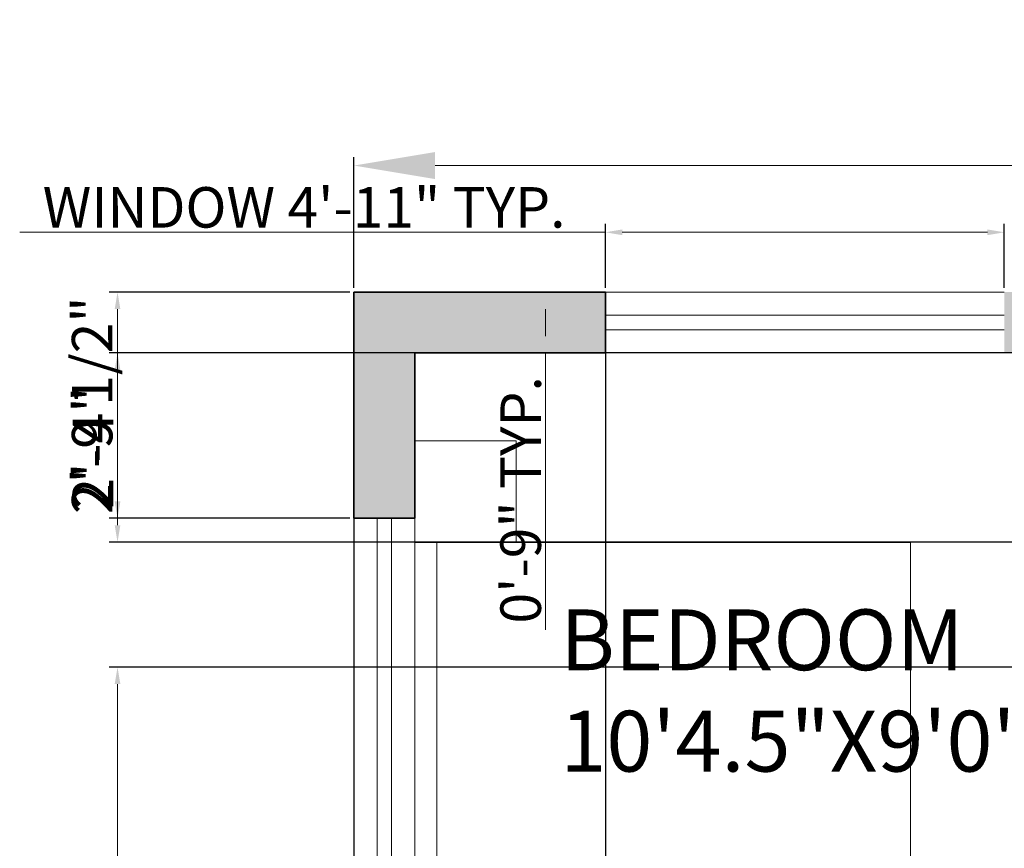
# Model space of a CAD drawing. Units: inches. Extents: x 2696 to 3240, y 1564 to 2310.
# Tile 53 of 76: x 2696 to 2842, y 2180 to 2303. Entities that reach past the tile are written whole.
import ezdxf

# ---------------------------------------------------------------- set-up
doc = ezdxf.new("R2010")
doc.units = ezdxf.units.IN
for name, color, linetype, lineweight in [('A-ANNO-DIMS', 3, 'Continuous', 18), ('A-AREA-IDEN', 7, 'Continuous', 18), ('A-FURN', 251, 'Continuous', 13), ('A-WALL', 7, 'Continuous', 35), ('A-WALL-PATT', 9, 'Continuous', 13), ('WINDOW', 2, 'Continuous', 18)]:
    doc.layers.add(name, color=color, linetype=linetype, lineweight=lineweight)
doc.styles.add('TIMES NEW', font='times.ttf')
doc.styles.add('YQ_DIM', font='SUPEROS.SHX', dxfattribs={"width": 0.8, "bigfont": 'HZDX.SHX'})
doc.dimstyles.new('Siddhuu', dxfattribs={"dimtxt": 6, "dimasz": 2.5, "dimexe": 1.25, "dimexo": 0.625, "dimtad": 1, "dimdec": 1, "dimlunit": 4, "dimtxsty": 'TIMES NEW', "dimcen": 2.5, "dimclrd": 256, "dimclre": 1, "dimclrt": 7, "dimadec": 0, "dimazin": 0, "dimtfac": 1, "dimtdec": 1, "dimtmove": 0, "dimatfit": 3, "dimfxl": 1, "dimtolj": 1, "dimlwd": -1, "dimarcsym": 0})

# ---------------------------------------------------------------- blocks, each defined once
blk = doc.blocks.new('WD_WIN4')
for p, q in [((-0.5, 0.5), (0.5, 0.5)), ((-0.5, 0.12), (0.5, 0.12)), ((-0.5, -0.12), (0.5, -0.12)), ((-0.5, -0.5), (0.5, -0.5))]:
    blk.add_line(p, q)
blk = doc.blocks.new('*D9')
at = {"layer": 'A-ANNO-DIMS', "color": 0, "lineweight": -2, "transparency": 16777216}
for p, q in [((2745.61, 2262.83), (2745.61, 2282.19)), ((3199.61, 2262.83), (3199.61, 2282.19))]:
    blk.add_line(p, q, dxfattribs=at)
at = {"layer": 'A-ANNO-DIMS', "color": 0, "transparency": 16777216}
blk.add_line((2757.61, 2280.94), (3187.61, 2280.94), dxfattribs=at)
for points in [[(2757.61, 2282.94), (2757.61, 2278.94), (2745.61, 2280.94)], [(3187.61, 2282.94), (3187.61, 2278.94), (3199.61, 2280.94)]]:
    blk.add_solid(points, dxfattribs=at)
at = {"layer": 'Defpoints', "color": 0, "transparency": 16777216}
for p in [(3199.61, 2280.94), (2745.61, 2262.2), (3199.61, 2262.2)]:
    blk.add_point(p, dxfattribs=at)
at = {"layer": 'A-ANNO-DIMS', "color": 0, "transparency": 16777216, "insert": (2972.61, 2290.72), "char_height": 18, "attachment_point": 5, "style": 'TIMES NEW'}
blk.add_mtext("\\A1;36'", dxfattribs=at)
blk = doc.blocks.new('BED-DOUBLE-WITH-NIGHTSTANDS')
for points in [[(0, 75.13), (0, 90.16), (15.03, 90.16), (15.03, 75.13)], [(3.28, 15.03), (3.28, 75.13), (73.4, 75.13), (73.4, 15.03)], [(0, 15.03), (0, 0), (15.03, 0), (15.03, 15.03)]]:
    blk.add_lwpolyline(points, close=True)
blk = doc.blocks.new('*D18')
at = {"layer": 'A-ANNO-DIMS', "transparency": 16777216}
for p, q in [((2782.83, 2271.06), (2696.13, 2271.06)), ((2839.39, 2271.06), (2785.33, 2271.06))]:
    blk.add_line(p, q, dxfattribs=at)
at = {"layer": 'A-ANNO-DIMS', "color": 1, "lineweight": -2, "transparency": 16777216}
for p, q in [((2782.83, 2262.83), (2782.83, 2272.31)), ((2841.89, 2262.83), (2841.89, 2272.31))]:
    blk.add_line(p, q, dxfattribs=at)
at = {"layer": 'A-ANNO-DIMS', "transparency": 16777216}
for points in [[(2785.33, 2271.48), (2785.33, 2270.64), (2782.83, 2271.06)], [(2839.39, 2271.48), (2839.39, 2270.64), (2841.89, 2271.06)]]:
    blk.add_solid(points, dxfattribs=at)
at = {"layer": 'Defpoints', "color": 0, "transparency": 16777216}
for p in [(2782.83, 2271.06), (2782.83, 2262.2), (2841.89, 2262.2)]:
    blk.add_point(p, dxfattribs=at)
at = {"layer": 'A-ANNO-DIMS', "color": 7, "transparency": 16777216, "insert": (2738.23, 2274.75), "char_height": 6, "attachment_point": 5, "style": 'TIMES NEW'}
blk.add_mtext('\\A1;WINDOW 4\'-11" TYP.', dxfattribs=at)
blk = doc.blocks.new('*D19')
at = {"layer": 'A-ANNO-DIMS', "color": 1, "lineweight": -2, "transparency": 16777216}
for p, q in [((2782.21, 2262.2), (2772.73, 2262.2)), ((2782.21, 2253.2), (2772.73, 2253.2))]:
    blk.add_line(p, q, dxfattribs=at)
at = {"layer": 'A-ANNO-DIMS', "transparency": 16777216}
for p, q in [((2773.98, 2259.7), (2773.98, 2255.7)), ((2773.98, 2253.2), (2773.98, 2212.21))]:
    blk.add_line(p, q, dxfattribs=at)
for points in [[(2773.56, 2259.7), (2774.39, 2259.7), (2773.98, 2262.2)], [(2773.56, 2255.7), (2774.39, 2255.7), (2773.98, 2253.2)]]:
    blk.add_solid(points, dxfattribs=at)
at = {"layer": 'Defpoints', "color": 0, "transparency": 16777216}
for p in [(2782.83, 2262.2), (2773.98, 2253.2), (2782.83, 2253.2)]:
    blk.add_point(p, dxfattribs=at)
at = {"layer": 'A-ANNO-DIMS', "color": 7, "transparency": 16777216, "insert": (2770.29, 2231.46), "char_height": 6, "attachment_point": 5, "rotation": 90, "style": 'TIMES NEW'}
blk.add_mtext('\\A1;0\'-9" TYP.', dxfattribs=at)
blk = doc.blocks.new('*D64')
at = {"layer": 'A-ANNO-DIMS', "color": 1, "lineweight": -2, "transparency": 16777216}
for p, q in [((3073.08, 2206.7), (2709.36, 2206.7)), ((3068.58, 1989.2), (2709.36, 1989.2))]:
    blk.add_line(p, q, dxfattribs=at)
at = {"layer": 'A-ANNO-DIMS', "transparency": 16777216}
blk.add_line((2710.61, 1991.7), (2710.61, 2204.2), dxfattribs=at)
for points in [[(2710.19, 2204.2), (2711.03, 2204.2), (2710.61, 2206.7)], [(2710.19, 1991.7), (2711.03, 1991.7), (2710.61, 1989.2)]]:
    blk.add_solid(points, dxfattribs=at)
at = {"layer": 'Defpoints', "color": 0, "transparency": 16777216}
for p in [(2710.61, 2206.7), (3073.71, 2206.7), (3069.21, 1989.2)]:
    blk.add_point(p, dxfattribs=at)
at = {"layer": 'A-ANNO-DIMS', "color": 7, "transparency": 16777216, "insert": (2706.85, 2097.95), "char_height": 6, "attachment_point": 5, "rotation": 90, "style": 'TIMES NEW'}
blk.add_mtext('\\A1;18\'-1 1/2"', dxfattribs=at)
blk = doc.blocks.new('*D68')
at = {"layer": 'A-ANNO-DIMS', "color": 1, "lineweight": -2, "transparency": 16777216}
for p, q in [((2745.61, 2261.58), (2745.61, 1568.95)), ((2782.83, 2261.58), (2782.83, 1568.95))]:
    blk.add_line(p, q, dxfattribs=at)
at = {"layer": 'A-ANNO-DIMS', "transparency": 16777216}
blk.add_line((2748.11, 1570.2), (2780.33, 1570.2), dxfattribs=at)
for points in [[(2748.11, 1570.62), (2748.11, 1569.78), (2745.61, 1570.2)], [(2780.33, 1570.62), (2780.33, 1569.78), (2782.83, 1570.2)]]:
    blk.add_solid(points, dxfattribs=at)
at = {"layer": 'Defpoints', "color": 0, "transparency": 16777216}
for p in [(2745.61, 2262.2), (2782.83, 2262.2), (2782.83, 1570.2)]:
    blk.add_point(p, dxfattribs=at)
at = {"layer": 'A-ANNO-DIMS', "color": 7, "transparency": 16777216, "insert": (2764.22, 1573.88), "char_height": 6, "attachment_point": 5, "style": 'TIMES NEW'}
blk.add_mtext('\\A1;3\'-1"', dxfattribs=at)
blk = doc.blocks.new('*D71')
at = {"layer": 'A-ANNO-DIMS', "color": 1, "lineweight": -2, "transparency": 16777216}
for p, q in [((2744.99, 2262.2), (2709.36, 2262.2)), ((2744.99, 2228.73), (2709.36, 2228.73))]:
    blk.add_line(p, q, dxfattribs=at)
at = {"layer": 'A-ANNO-DIMS', "transparency": 16777216}
blk.add_line((2710.61, 2259.7), (2710.61, 2231.23), dxfattribs=at)
for points in [[(2710.19, 2259.7), (2711.03, 2259.7), (2710.61, 2262.2)], [(2710.19, 2231.23), (2711.03, 2231.23), (2710.61, 2228.73)]]:
    blk.add_solid(points, dxfattribs=at)
at = {"layer": 'Defpoints', "color": 0, "transparency": 16777216}
for p in [(2745.61, 2262.2), (2710.61, 2228.73), (2745.61, 2228.73)]:
    blk.add_point(p, dxfattribs=at)
at = {"layer": 'A-ANNO-DIMS', "color": 7, "transparency": 16777216, "insert": (2706.85, 2245.46), "char_height": 6, "attachment_point": 5, "rotation": 90, "style": 'TIMES NEW'}
blk.add_mtext('\\A1;2\'-9 1/2"', dxfattribs=at)
blk = doc.blocks.new('*D76')
at = {"layer": 'A-ANNO-DIMS', "color": 1, "lineweight": -2, "transparency": 16777216}
for p, q in [((3189.99, 2253.2), (2709.36, 2253.2)), ((3189.99, 2225.2), (2709.36, 2225.2))]:
    blk.add_line(p, q, dxfattribs=at)
at = {"layer": 'A-ANNO-DIMS', "transparency": 16777216}
blk.add_line((2710.61, 2250.7), (2710.61, 2227.7), dxfattribs=at)
for points in [[(2710.19, 2250.7), (2711.03, 2250.7), (2710.61, 2253.2)], [(2710.19, 2227.7), (2711.03, 2227.7), (2710.61, 2225.2)]]:
    blk.add_solid(points, dxfattribs=at)
at = {"layer": 'Defpoints', "color": 0, "transparency": 16777216}
for p in [(3190.61, 2253.2), (2710.61, 2225.2), (3190.61, 2225.2)]:
    blk.add_point(p, dxfattribs=at)
at = {"layer": 'A-ANNO-DIMS', "color": 7, "transparency": 16777216, "insert": (2706.99, 2239.2), "char_height": 6, "attachment_point": 5, "rotation": 90, "style": 'TIMES NEW'}
blk.add_mtext('\\A1;2\'-4"', dxfattribs=at)

msp = doc.modelspace()

# ---------------------------------------------------------------- hatches: boundary and pattern name
at = {"layer": 'A-WALL-PATT', "transparency": 33554556}
h = msp.add_hatch(color=256, dxfattribs=at)
h.dxf.hatch_style = 1
h.paths.add_polyline_path([(2879.11, 2253.2), (2905.91, 2253.2), (2905.91, 2262.2), (2841.89, 2262.2), (2841.89, 2253.2), (2870.11, 2253.2), (2870.11, 2176.6), (2965.71, 2176.6), (2965.71, 2206.7), (2973.58, 2206.7), (2973.58, 2215.7), (2965.71, 2215.7), (2965.71, 2262.2), (2929.91, 2262.2), (2929.91, 2253.2), (2956.71, 2253.2), (2956.71, 2185.6), (2879.11, 2185.6)])
h.paths.add_polyline_path([(2782.83, 2262.2), (2745.61, 2262.2), (2745.61, 2228.73), (2754.61, 2228.73), (2754.61, 2253.2), (2782.83, 2253.2)])
h.paths.add_polyline_path([(2754.61, 2136.2), (2965.71, 2136.2), (2965.71, 2145.2), (2879.11, 2145.2), (2879.11, 2147.07), (2877.34, 2147.07), (2870.11, 2147.07), (2870.11, 2145.2), (2754.61, 2145.2), (2754.61, 2169.67), (2745.61, 2169.67), (2745.61, 2000.2), (2754.61, 2000.2), (2754.61, 2019.2), (2849.08, 2019.2), (2849.08, 2023.7), (2841.21, 2023.7), (2841.21, 2051.83), (2836.71, 2051.83), (2836.71, 2023.7), (2754.61, 2023.7), (2754.61, 2091.2), (2836.71, 2091.2), (2836.71, 2087.83), (2841.21, 2087.83), (2841.21, 2095.7), (2754.61, 2095.7)])
h.paths.add_polyline_path([(2965.71, 2136.2), (2956.71, 2136.2), (2956.71, 2023.7), (2885.08, 2023.7), (2885.08, 2019.2), (2956.71, 2019.2), (2956.71, 1950.58), (2965.71, 1950.58), (2965.71, 1980.2), (2973.58, 1980.2), (2973.58, 1989.2), (2965.71, 1989.2)])
h.paths.add_polyline_path([(2754.61, 1906.7), (2880.21, 1906.7), (2884.71, 1906.7), (2956.71, 1906.7), (2956.71, 1792.7), (2944.71, 1792.7), (2944.71, 1783.7), (2956.71, 1783.7), (2956.71, 1740.2), (2884.71, 1740.2), (2884.71, 1783.7), (2896.71, 1783.7), (2896.71, 1792.7), (2884.71, 1792.7), (2884.71, 1846.7), (2880.21, 1846.7), (2880.21, 1740.2), (2754.61, 1740.2), (2754.61, 1777.2), (2745.61, 1777.2), (2745.61, 1692.7), (2754.61, 1692.7), (2754.61, 1731.2), (2956.71, 1731.2), (2956.71, 1723.33), (2965.71, 1723.33), (2965.71, 1884.2), (2973.58, 1884.2), (2973.58, 1893.2), (2965.71, 1893.2), (2965.71, 1914.58), (2956.71, 1914.58), (2956.71, 1911.2), (2754.61, 1911.2), (2754.61, 1930.2), (2745.61, 1930.2), (2745.61, 1817.2), (2754.61, 1817.2), (2754.61, 1854.2), (2826.61, 1854.2), (2826.61, 1868.83), (2822.11, 1868.83), (2822.11, 1858.7), (2754.61, 1858.7)])
h.paths.add_polyline_path([(2965.71, 1656.2), (3008.24, 1656.2), (3008.24, 1665.2), (2965.71, 1665.2), (2965.71, 1693.33), (2956.71, 1693.33), (2956.71, 1686.2), (2934.58, 1686.2), (2934.58, 1681.7), (2956.71, 1681.7), (2956.71, 1614.2), (2896.71, 1614.2), (2896.71, 1681.7), (2904.58, 1681.7), (2904.58, 1686.2), (2892.21, 1686.2), (2892.21, 1614.2), (2858.41, 1614.2), (2858.41, 1605.2), (2965.71, 1605.2)])
h.paths.add_polyline_path([(2788.41, 1614.2), (2754.61, 1614.2), (2754.61, 1652.7), (2745.61, 1652.7), (2745.61, 1605.2), (2788.41, 1605.2)])
h.paths.add_polyline_path([(3199.61, 1633.05), (3190.61, 1633.05), (3190.61, 1614.2), (3082.61, 1614.2), (3082.61, 1665.2), (3070.24, 1665.2), (3070.24, 1656.2), (3078.11, 1656.2), (3078.11, 1605.2), (3199.61, 1605.2)])
h.paths.add_polyline_path([(3199.61, 1702.05), (3190.61, 1702.05), (3190.61, 1699.7), (3106.61, 1699.7), (3106.61, 1747.7), (3190.61, 1747.7), (3190.61, 1752.2), (3082.61, 1752.2), (3082.61, 1760.08), (3078.11, 1760.08), (3078.11, 1747.7), (3102.11, 1747.7), (3102.11, 1699.7), (3078.11, 1699.7), (3078.11, 1695.2), (3190.61, 1695.2), (3190.61, 1676.35), (3199.61, 1676.35)])
h.paths.add_polyline_path([(3199.61, 1783.2), (3190.61, 1783.2), (3190.61, 1745.35), (3199.61, 1745.35)])
h.paths.add_polyline_path([(3082.61, 1884.2), (3190.61, 1884.2), (3190.61, 1853.2), (3199.61, 1853.2), (3199.61, 1901.7), (3190.61, 1901.7), (3190.61, 1893.2), (3005.58, 1893.2), (3005.58, 1891.28), (3005.58, 1884.2), (3078.11, 1884.2), (3078.11, 1792.08), (3082.61, 1792.08)])
h.paths.add_polyline_path([(3199.61, 1994.7), (3190.61, 1994.7), (3190.61, 1989.2), (3073.71, 1989.2), (3073.71, 2034.2), (3069.21, 2034.2), (3069.21, 1989.2), (3005.58, 1989.2), (3005.58, 1980.2), (3190.61, 1980.2), (3190.61, 1971.7), (3199.61, 1971.7)])
h.paths.add_polyline_path([(3199.61, 2155.2), (3190.61, 2155.2), (3190.61, 2064.7), (3199.61, 2064.7)])
h.paths.add_polyline_path([(3190.61, 2074.7), (3106.61, 2074.7), (3106.61, 2122.7), (3190.61, 2122.7), (3190.61, 2127.2), (3082.71, 2127.2), (3082.71, 2135.08), (3073.71, 2135.08), (3073.71, 2122.7), (3102.11, 2122.7), (3102.11, 2074.7), (3069.21, 2074.7), (3069.21, 2070.2), (3190.61, 2070.2)])
h.paths.add_polyline_path([(3082.71, 2253.2), (3190.61, 2253.2), (3190.61, 2225.2), (3199.61, 2225.2), (3199.61, 2262.2), (3073.71, 2262.2), (3073.71, 2215.7), (3035.58, 2215.7), (3035.58, 2206.7), (3073.71, 2206.7), (3073.71, 2171.08), (3082.71, 2171.08)])

# ---------------------------------------------------------------- linework, layer by layer
at = {"layer": 'A-WALL'}
for p, q in [((2745.61, 2262.2), (2782.83, 2262.2)), ((2745.61, 2228.73), (2745.61, 2262.2)), ((2782.83, 2253.2), (2782.83, 2262.2)), ((2754.61, 2253.2), (2782.83, 2253.2)), ((2754.61, 2228.73), (2754.61, 2253.2)), ((2754.61, 2228.73), (2745.61, 2228.73))]:
    msp.add_line(p, q, dxfattribs=at)

# ---------------------------------------------------------------- block references
at = {"layer": 'A-FURN'}
msp.add_blockref('BED-DOUBLE-WITH-NIGHTSTANDS', (2754.61, 2150.02), dxfattribs=at)
at = {"layer": 'WINDOW', "xscale": 59.05511811023622, "zscale": 59.05511811023622}
for p, yscale, rotation in [((2812.36, 2257.7), 9.000000000000455, 180.0000000000004), ((2750.11, 2199.2), 8.999999999999545, 269.9999999999996)]:
    msp.add_blockref('WD_WIN4', p, dxfattribs=dict(at, yscale=yscale, rotation=rotation))

# ---------------------------------------------------------------- texts
at = {"layer": 'A-AREA-IDEN', "insert": (2776.16, 2215.24), "char_height": 9, "attachment_point": 1, "style": 'YQ_DIM'}
msp.add_mtext_dynamic_manual_height_columns('BEDROOM\\P10\'4.5"X9\'0"', width=48.0032, gutter_width=12.5, heights=[0], dxfattribs=at)

# ---------------------------------------------------------------- dimensions: what is measured, and where the dimension line sits
at = {"layer": 'A-ANNO-DIMS'}
dim = msp.add_linear_dim(base=(3199.61, 2280.94), p1=(2745.61, 2262.2), p2=(3199.61, 2262.2), text="36'", dimstyle='Siddhuu', override={"dimtxt": 18, "dimasz": 12, "dimclrd": 0, "dimclre": 0, "dimclrt": 0}, dxfattribs=at)
dim.commit()
dim.dimension.update_dxf_attribs({"geometry": '*D9', "text_midpoint": (2972.61, 2290.72)})
for base, p1, p2, angle, text, picture, middle in [((2782.83, 2271.06), (2841.89, 2262.2), (2782.83, 2262.2), 180, 'WINDOW <> TYP.', '*D18', (2738.23, 2274.75)), ((2773.98, 2253.2), (2782.83, 2262.2), (2782.83, 2253.2), 270, '<> TYP.', '*D19', (2770.29, 2231.46))]:
    dim = msp.add_linear_dim(base=base, p1=p1, p2=p2, angle=angle, text=text, dimstyle='Siddhuu', override={"dimdec": 1, "dimlfac": 1, "dimrnd": 0, "dimzin": 1, "dimdsep": 46, "dimlunit": 4, "dimfrac": 2}, dxfattribs=at)
    dim.commit()
    dim.dimension.update_dxf_attribs({"geometry": picture, "text_midpoint": middle})
for base, p1, p2, picture, middle in [((2710.61, 2228.73), (2745.61, 2262.2), (2745.61, 2228.73), '*D71', (2706.85, 2245.46)), ((2710.61, 2225.2), (3190.61, 2253.2), (3190.61, 2225.2), '*D76', (2706.99, 2239.2)), ((2710.61, 2206.7), (3069.21, 1989.2), (3073.71, 2206.7), '*D64', (2706.85, 2097.95))]:
    dim = msp.add_linear_dim(base=base, p1=p1, p2=p2, angle=90, dimstyle='Siddhuu', override={"dimdec": 1, "dimlfac": 1, "dimrnd": 0, "dimzin": 1, "dimdsep": 46, "dimlunit": 4, "dimfrac": 2}, dxfattribs=at)
    dim.commit()
    dim.dimension.update_dxf_attribs({"geometry": picture, "text_midpoint": middle})
dim = msp.add_linear_dim(base=(2782.83, 1570.2), p1=(2745.61, 2262.2), p2=(2782.83, 2262.2), dimstyle='Siddhuu', override={"dimdec": 1, "dimlfac": 1, "dimrnd": 0, "dimzin": 1, "dimdsep": 46, "dimlunit": 4, "dimfrac": 2}, dxfattribs=at)
dim.commit()
dim.dimension.update_dxf_attribs({"geometry": '*D68', "text_midpoint": (2764.22, 1573.88)})

doc.saveas('drawing.dxf')
